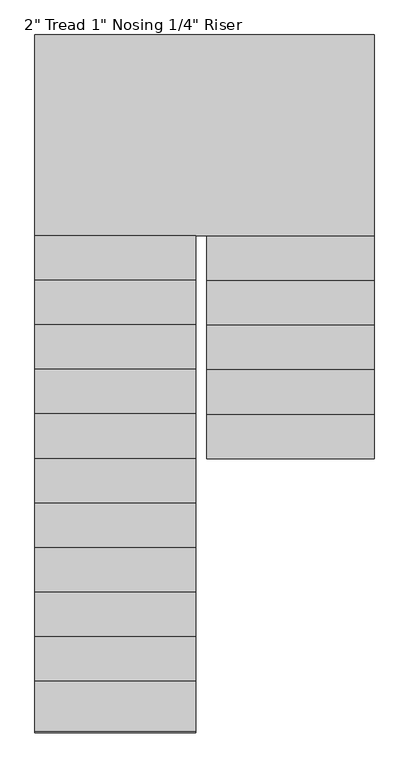
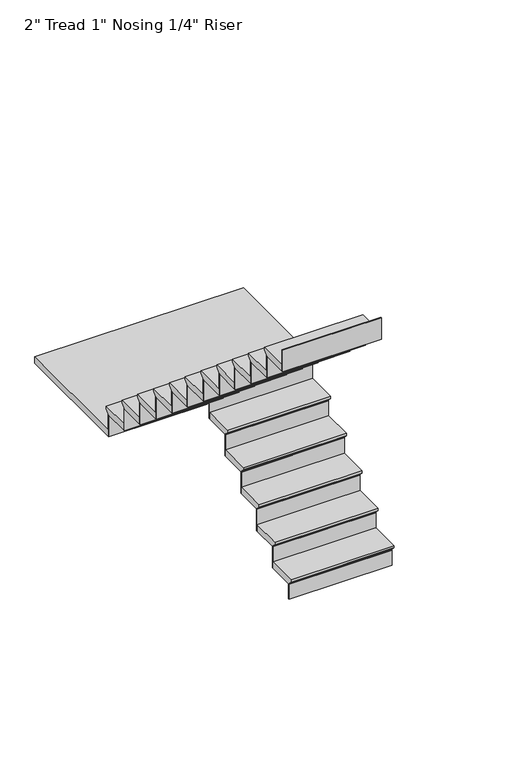
"""IFC4 building model written with IfcOpenShell, lengths in millimetres: stair flight geometry."""

from ifc_helpers import new_model, si_unit, origin, place, context, project, spatial, faceted_brep, source, transform, mapped, element, save


def stair_flight_e13e2030(model_context):
    return source(origin(), model_context, "Body", "Brep", [
        faceted_brep([(-3749.597125, 2714.6319226, 9141.8833333), (-3749.597125, 2714.6319226, 9160.9333333), (-4512.2136682, 2714.6319226, 9160.9333333), (-4512.2136682, 2714.6319226, 9141.8833333), (-3749.597125, 2740.0319226, 9116.4833333), (-4512.2136682, 2740.0319226, 9116.4833333), (-3749.597125, 2943.2319226, 9160.9333333), (-4512.2136682, 2943.2319226, 9160.9333333), (-4512.2136682, 2740.0319226, 9110.1333333), (-4512.2136682, 2943.2319226, 9110.1333333), (-3749.597125, 2943.2319226, 9110.1333333), (-3749.597125, 2740.0319226, 9110.1333333)], [[[0, 1, 2, 3]], [[4, 0, 3, 5]], [[2, 1, 6, 7]], [[8, 9, 10, 11]], [[2, 7, 9, 8, 5, 3]], [[8, 11, 4, 5]], [[6, 1, 0, 4, 11, 10]], [[7, 6, 10, 9]]]),
        faceted_brep([(-3749.597125, 2740.0319226, 9110.1333333), (-3749.597125, 2740.0319226, 8991.6), (-3749.597125, 2746.3819226, 8991.6), (-3749.597125, 2746.3819226, 9110.1333333), (-4512.2136682, 2740.0319226, 9110.1333333), (-4512.2136682, 2746.3819226, 9110.1333333), (-4512.2136682, 2746.3819226, 8991.6), (-4512.2136682, 2740.0319226, 8991.6)], [[[0, 1, 2, 3]], [[4, 5, 6, 7]], [[1, 0, 4, 7]], [[2, 1, 7, 6]], [[3, 2, 6, 5]], [[0, 3, 5, 4]]]),
        faceted_brep([(-3749.597125, 2943.2319226, 9279.4666667), (-3749.597125, 2943.2319226, 9110.1333333), (-3749.597125, 2949.5819226, 9110.1333333), (-3749.597125, 2949.5819226, 9279.4666667), (-4512.2136682, 2943.2319226, 9279.4666667), (-4512.2136682, 2949.5819226, 9279.4666667), (-4512.2136682, 2949.5819226, 9110.1333333), (-4512.2136682, 2943.2319226, 9110.1333333)], [[[0, 1, 2, 3]], [[4, 5, 6, 7]], [[1, 0, 4, 7]], [[2, 1, 7, 6]], [[3, 2, 6, 5]], [[0, 3, 5, 4]]]),
        faceted_brep([(-4512.2136682, 2917.8319226, 9330.2666667), (-3749.597125, 2917.8319226, 9330.2666667), (-3749.597125, 3146.4319226, 9330.2666667), (-4512.2136682, 3146.4319226, 9330.2666667), (-4512.2136682, 2943.2319226, 9279.4666667), (-4512.2136682, 3146.4319226, 9279.4666667), (-3749.597125, 3146.4319226, 9279.4666667), (-3749.597125, 2943.2319226, 9279.4666667), (-4512.2136682, 2943.2319226, 9285.8166667), (-4512.2136682, 2917.8319226, 9311.2166667), (-3749.597125, 2943.2319226, 9285.8166667), (-3749.597125, 2917.8319226, 9311.2166667)], [[[0, 1, 2, 3]], [[4, 5, 6, 7]], [[0, 3, 5, 4, 8, 9]], [[4, 7, 10, 8]], [[2, 1, 11, 10, 7, 6]], [[3, 2, 6, 5]], [[11, 1, 0, 9]], [[10, 11, 9, 8]]]),
        faceted_brep([(-3749.597125, 3146.4319226, 9448.8), (-3749.597125, 3146.4319226, 9279.4666667), (-3749.597125, 3152.7819226, 9279.4666667), (-3749.597125, 3152.7819226, 9448.8), (-4512.2136682, 3146.4319226, 9448.8), (-4512.2136682, 3152.7819226, 9448.8), (-4512.2136682, 3152.7819226, 9279.4666667), (-4512.2136682, 3146.4319226, 9279.4666667)], [[[0, 1, 2, 3]], [[4, 5, 6, 7]], [[1, 0, 4, 7]], [[2, 1, 7, 6]], [[3, 2, 6, 5]], [[0, 3, 5, 4]]]),
        faceted_brep([(-4512.2136682, 3121.0319226, 9499.6), (-3749.597125, 3121.0319226, 9499.6), (-3749.597125, 3349.6319226, 9499.6), (-4512.2136682, 3349.6319226, 9499.6), (-4512.2136682, 3146.4319226, 9448.8), (-4512.2136682, 3349.6319226, 9448.8), (-3749.597125, 3349.6319226, 9448.8), (-3749.597125, 3146.4319226, 9448.8), (-4512.2136682, 3146.4319226, 9455.15), (-4512.2136682, 3121.0319226, 9480.55), (-3749.597125, 3146.4319226, 9455.15), (-3749.597125, 3121.0319226, 9480.55)], [[[0, 1, 2, 3]], [[4, 5, 6, 7]], [[0, 3, 5, 4, 8, 9]], [[4, 7, 10, 8]], [[2, 1, 11, 10, 7, 6]], [[3, 2, 6, 5]], [[11, 1, 0, 9]], [[10, 11, 9, 8]]]),
        faceted_brep([(-3749.597125, 3349.6319226, 9618.1333333), (-3749.597125, 3349.6319226, 9448.8), (-3749.597125, 3355.9819226, 9448.8), (-3749.597125, 3355.9819226, 9618.1333333), (-4512.2136682, 3349.6319226, 9618.1333333), (-4512.2136682, 3355.9819226, 9618.1333333), (-4512.2136682, 3355.9819226, 9448.8), (-4512.2136682, 3349.6319226, 9448.8)], [[[0, 1, 2, 3]], [[4, 5, 6, 7]], [[1, 0, 4, 7]], [[2, 1, 7, 6]], [[3, 2, 6, 5]], [[0, 3, 5, 4]]]),
        faceted_brep([(-4512.2136682, 3324.2319226, 9668.9333333), (-3749.597125, 3324.2319226, 9668.9333333), (-3749.597125, 3552.8319226, 9668.9333333), (-4512.2136682, 3552.8319226, 9668.9333333), (-4512.2136682, 3349.6319226, 9618.1333333), (-4512.2136682, 3552.8319226, 9618.1333333), (-3749.597125, 3552.8319226, 9618.1333333), (-3749.597125, 3349.6319226, 9618.1333333), (-4512.2136682, 3349.6319226, 9624.4833333), (-4512.2136682, 3324.2319226, 9649.8833333), (-3749.597125, 3349.6319226, 9624.4833333), (-3749.597125, 3324.2319226, 9649.8833333)], [[[0, 1, 2, 3]], [[4, 5, 6, 7]], [[0, 3, 5, 4, 8, 9]], [[4, 7, 10, 8]], [[2, 1, 11, 10, 7, 6]], [[3, 2, 6, 5]], [[11, 1, 0, 9]], [[10, 11, 9, 8]]]),
        faceted_brep([(-3749.597125, 3552.8319226, 9787.4666667), (-3749.597125, 3552.8319226, 9618.1333333), (-3749.597125, 3559.1819226, 9618.1333333), (-3749.597125, 3559.1819226, 9787.4666667), (-4512.2136682, 3552.8319226, 9787.4666667), (-4512.2136682, 3559.1819226, 9787.4666667), (-4512.2136682, 3559.1819226, 9618.1333333), (-4512.2136682, 3552.8319226, 9618.1333333)], [[[0, 1, 2, 3]], [[4, 5, 6, 7]], [[1, 0, 4, 7]], [[2, 1, 7, 6]], [[3, 2, 6, 5]], [[0, 3, 5, 4]]]),
        faceted_brep([(-4512.2136682, 3527.4319226, 9838.2666667), (-3749.597125, 3527.4319226, 9838.2666667), (-3749.597125, 3756.0319226, 9838.2666667), (-4512.2136682, 3756.0319226, 9838.2666667), (-4512.2136682, 3552.8319226, 9787.4666667), (-4512.2136682, 3756.0319226, 9787.4666667), (-3749.597125, 3756.0319226, 9787.4666667), (-3749.597125, 3552.8319226, 9787.4666667), (-4512.2136682, 3552.8319226, 9793.8166667), (-4512.2136682, 3527.4319226, 9819.2166667), (-3749.597125, 3552.8319226, 9793.8166667), (-3749.597125, 3527.4319226, 9819.2166667)], [[[0, 1, 2, 3]], [[4, 5, 6, 7]], [[0, 3, 5, 4, 8, 9]], [[4, 7, 10, 8]], [[2, 1, 11, 10, 7, 6]], [[3, 2, 6, 5]], [[11, 1, 0, 9]], [[10, 11, 9, 8]]]),
        faceted_brep([(-3749.597125, 3756.0319226, 9956.8), (-3749.597125, 3756.0319226, 9787.4666667), (-3749.597125, 3762.3819226, 9787.4666667), (-3749.597125, 3762.3819226, 9956.8), (-4512.2136682, 3756.0319226, 9956.8), (-4512.2136682, 3762.3819226, 9956.8), (-4512.2136682, 3762.3819226, 9787.4666667), (-4512.2136682, 3756.0319226, 9787.4666667)], [[[0, 1, 2, 3]], [[4, 5, 6, 7]], [[1, 0, 4, 7]], [[2, 1, 7, 6]], [[3, 2, 6, 5]], [[0, 3, 5, 4]]]),
        faceted_brep([(-4563.0136682, 3705.2319226, 10007.6), (-4563.0136682, 3730.6319226, 10007.6), (-3749.597125, 3730.6319226, 10007.6), (-3749.597125, 4645.0319226, 10007.6), (-5295.0246464, 4645.0319226, 10007.6), (-5295.0246464, 3705.2319226, 10007.6), (-4563.0136682, 3730.6319226, 9956.8), (-4563.0136682, 3705.2319226, 9956.8), (-5295.0246464, 3705.2319226, 9956.8), (-5295.0246464, 4645.0319226, 9956.8), (-3749.597125, 4645.0319226, 9956.8), (-3749.597125, 3756.0319226, 9956.8), (-4512.2136682, 3756.0319226, 9956.8), (-4512.2136682, 3730.6319226, 9956.8), (-4512.2136682, 3730.6319226, 9988.55), (-3749.597125, 3730.6319226, 9988.55), (-4512.2136682, 3756.0319226, 9963.15), (-3749.597125, 3756.0319226, 9963.15)], [[[0, 1, 2, 3, 4, 5]], [[6, 7, 8, 9, 10, 11, 12, 13]], [[1, 0, 7, 6]], [[2, 1, 6, 13, 14, 15]], [[13, 12, 16, 14]], [[12, 11, 17, 16]], [[3, 2, 15, 17, 11, 10]], [[4, 3, 10, 9]], [[5, 4, 9, 8]], [[0, 5, 8, 7]], [[17, 15, 14, 16]]]),
        faceted_brep([(-5295.0246464, 3705.2319226, 10126.1333333), (-5295.0246464, 3705.2319226, 9956.8), (-5295.0246464, 3698.8819226, 9956.8), (-5295.0246464, 3698.8819226, 10126.1333333), (-4563.0136682, 3705.2319226, 10126.1333333), (-4563.0136682, 3698.8819226, 10126.1333333), (-4563.0136682, 3698.8819226, 9956.8), (-4563.0136682, 3705.2319226, 9956.8)], [[[0, 1, 2, 3]], [[4, 5, 6, 7]], [[1, 0, 4, 7]], [[2, 1, 7, 6]], [[3, 2, 6, 5]], [[0, 3, 5, 4]]]),
        faceted_brep([(-4563.0136682, 3730.6319226, 10176.9333333), (-5295.0246464, 3730.6319226, 10176.9333333), (-5295.0246464, 3502.0319226, 10176.9333333), (-4563.0136682, 3502.0319226, 10176.9333333), (-4563.0136682, 3705.2319226, 10126.1333333), (-4563.0136682, 3502.0319226, 10126.1333333), (-5295.0246464, 3502.0319226, 10126.1333333), (-5295.0246464, 3705.2319226, 10126.1333333), (-4563.0136682, 3705.2319226, 10132.4833333), (-4563.0136682, 3730.6319226, 10157.8833333), (-5295.0246464, 3705.2319226, 10132.4833333), (-5295.0246464, 3730.6319226, 10157.8833333)], [[[0, 1, 2, 3]], [[4, 5, 6, 7]], [[0, 3, 5, 4, 8, 9]], [[4, 7, 10, 8]], [[2, 1, 11, 10, 7, 6]], [[3, 2, 6, 5]], [[11, 1, 0, 9]], [[10, 11, 9, 8]]]),
        faceted_brep([(-5295.0246464, 3502.0319226, 10295.4666667), (-5295.0246464, 3502.0319226, 10126.1333333), (-5295.0246464, 3495.6819226, 10126.1333333), (-5295.0246464, 3495.6819226, 10295.4666667), (-4563.0136682, 3502.0319226, 10295.4666667), (-4563.0136682, 3495.6819226, 10295.4666667), (-4563.0136682, 3495.6819226, 10126.1333333), (-4563.0136682, 3502.0319226, 10126.1333333)], [[[0, 1, 2, 3]], [[4, 5, 6, 7]], [[1, 0, 4, 7]], [[2, 1, 7, 6]], [[3, 2, 6, 5]], [[0, 3, 5, 4]]]),
        faceted_brep([(-4563.0136682, 3527.4319226, 10346.2666667), (-5295.0246464, 3527.4319226, 10346.2666667), (-5295.0246464, 3298.8319226, 10346.2666667), (-4563.0136682, 3298.8319226, 10346.2666667), (-4563.0136682, 3502.0319226, 10295.4666667), (-4563.0136682, 3298.8319226, 10295.4666667), (-5295.0246464, 3298.8319226, 10295.4666667), (-5295.0246464, 3502.0319226, 10295.4666667), (-4563.0136682, 3502.0319226, 10301.8166667), (-4563.0136682, 3527.4319226, 10327.2166667), (-5295.0246464, 3502.0319226, 10301.8166667), (-5295.0246464, 3527.4319226, 10327.2166667)], [[[0, 1, 2, 3]], [[4, 5, 6, 7]], [[0, 3, 5, 4, 8, 9]], [[4, 7, 10, 8]], [[2, 1, 11, 10, 7, 6]], [[3, 2, 6, 5]], [[11, 1, 0, 9]], [[10, 11, 9, 8]]]),
        faceted_brep([(-5295.0246464, 3298.8319226, 10464.8), (-5295.0246464, 3298.8319226, 10295.4666667), (-5295.0246464, 3292.4819226, 10295.4666667), (-5295.0246464, 3292.4819226, 10464.8), (-4563.0136682, 3298.8319226, 10464.8), (-4563.0136682, 3292.4819226, 10464.8), (-4563.0136682, 3292.4819226, 10295.4666667), (-4563.0136682, 3298.8319226, 10295.4666667)], [[[0, 1, 2, 3]], [[4, 5, 6, 7]], [[1, 0, 4, 7]], [[2, 1, 7, 6]], [[3, 2, 6, 5]], [[0, 3, 5, 4]]]),
        faceted_brep([(-4563.0136682, 3324.2319226, 10515.6), (-5295.0246464, 3324.2319226, 10515.6), (-5295.0246464, 3095.6319226, 10515.6), (-4563.0136682, 3095.6319226, 10515.6), (-4563.0136682, 3298.8319226, 10464.8), (-4563.0136682, 3095.6319226, 10464.8), (-5295.0246464, 3095.6319226, 10464.8), (-5295.0246464, 3298.8319226, 10464.8), (-4563.0136682, 3298.8319226, 10471.15), (-4563.0136682, 3324.2319226, 10496.55), (-5295.0246464, 3298.8319226, 10471.15), (-5295.0246464, 3324.2319226, 10496.55)], [[[0, 1, 2, 3]], [[4, 5, 6, 7]], [[0, 3, 5, 4, 8, 9]], [[4, 7, 10, 8]], [[2, 1, 11, 10, 7, 6]], [[3, 2, 6, 5]], [[11, 1, 0, 9]], [[10, 11, 9, 8]]]),
        faceted_brep([(-5295.0246464, 3095.6319226, 10634.1333333), (-5295.0246464, 3095.6319226, 10464.8), (-5295.0246464, 3089.2819226, 10464.8), (-5295.0246464, 3089.2819226, 10634.1333333), (-4563.0136682, 3095.6319226, 10634.1333333), (-4563.0136682, 3089.2819226, 10634.1333333), (-4563.0136682, 3089.2819226, 10464.8), (-4563.0136682, 3095.6319226, 10464.8)], [[[0, 1, 2, 3]], [[4, 5, 6, 7]], [[1, 0, 4, 7]], [[2, 1, 7, 6]], [[3, 2, 6, 5]], [[0, 3, 5, 4]]]),
        faceted_brep([(-4563.0136682, 3121.0319226, 10684.9333333), (-5295.0246464, 3121.0319226, 10684.9333333), (-5295.0246464, 2892.4319226, 10684.9333333), (-4563.0136682, 2892.4319226, 10684.9333333), (-4563.0136682, 3095.6319226, 10634.1333333), (-4563.0136682, 2892.4319226, 10634.1333333), (-5295.0246464, 2892.4319226, 10634.1333333), (-5295.0246464, 3095.6319226, 10634.1333333), (-4563.0136682, 3095.6319226, 10640.4833333), (-4563.0136682, 3121.0319226, 10665.8833333), (-5295.0246464, 3095.6319226, 10640.4833333), (-5295.0246464, 3121.0319226, 10665.8833333)], [[[0, 1, 2, 3]], [[4, 5, 6, 7]], [[0, 3, 5, 4, 8, 9]], [[4, 7, 10, 8]], [[2, 1, 11, 10, 7, 6]], [[3, 2, 6, 5]], [[11, 1, 0, 9]], [[10, 11, 9, 8]]]),
        faceted_brep([(-5295.0246464, 2892.4319226, 10803.4666667), (-5295.0246464, 2892.4319226, 10634.1333333), (-5295.0246464, 2886.0819226, 10634.1333333), (-5295.0246464, 2886.0819226, 10803.4666667), (-4563.0136682, 2892.4319226, 10803.4666667), (-4563.0136682, 2886.0819226, 10803.4666667), (-4563.0136682, 2886.0819226, 10634.1333333), (-4563.0136682, 2892.4319226, 10634.1333333)], [[[0, 1, 2, 3]], [[4, 5, 6, 7]], [[1, 0, 4, 7]], [[2, 1, 7, 6]], [[3, 2, 6, 5]], [[0, 3, 5, 4]]]),
        faceted_brep([(-4563.0136682, 2917.8319226, 10854.2666667), (-5295.0246464, 2917.8319226, 10854.2666667), (-5295.0246464, 2689.2319226, 10854.2666667), (-4563.0136682, 2689.2319226, 10854.2666667), (-4563.0136682, 2892.4319226, 10803.4666667), (-4563.0136682, 2689.2319226, 10803.4666667), (-5295.0246464, 2689.2319226, 10803.4666667), (-5295.0246464, 2892.4319226, 10803.4666667), (-4563.0136682, 2892.4319226, 10809.8166667), (-4563.0136682, 2917.8319226, 10835.2166667), (-5295.0246464, 2892.4319226, 10809.8166667), (-5295.0246464, 2917.8319226, 10835.2166667)], [[[0, 1, 2, 3]], [[4, 5, 6, 7]], [[0, 3, 5, 4, 8, 9]], [[4, 7, 10, 8]], [[2, 1, 11, 10, 7, 6]], [[3, 2, 6, 5]], [[11, 1, 0, 9]], [[10, 11, 9, 8]]]),
        faceted_brep([(-5295.0246464, 2689.2319226, 10972.8), (-5295.0246464, 2689.2319226, 10803.4666667), (-5295.0246464, 2682.8819226, 10803.4666667), (-5295.0246464, 2682.8819226, 10972.8), (-4563.0136682, 2689.2319226, 10972.8), (-4563.0136682, 2682.8819226, 10972.8), (-4563.0136682, 2682.8819226, 10803.4666667), (-4563.0136682, 2689.2319226, 10803.4666667)], [[[0, 1, 2, 3]], [[4, 5, 6, 7]], [[1, 0, 4, 7]], [[2, 1, 7, 6]], [[3, 2, 6, 5]], [[0, 3, 5, 4]]]),
        faceted_brep([(-4563.0136682, 2714.6319226, 11023.6), (-5295.0246464, 2714.6319226, 11023.6), (-5295.0246464, 2486.0319226, 11023.6), (-4563.0136682, 2486.0319226, 11023.6), (-4563.0136682, 2689.2319226, 10972.8), (-4563.0136682, 2486.0319226, 10972.8), (-5295.0246464, 2486.0319226, 10972.8), (-5295.0246464, 2689.2319226, 10972.8), (-4563.0136682, 2689.2319226, 10979.15), (-4563.0136682, 2714.6319226, 11004.55), (-5295.0246464, 2689.2319226, 10979.15), (-5295.0246464, 2714.6319226, 11004.55)], [[[0, 1, 2, 3]], [[4, 5, 6, 7]], [[0, 3, 5, 4, 8, 9]], [[4, 7, 10, 8]], [[2, 1, 11, 10, 7, 6]], [[3, 2, 6, 5]], [[11, 1, 0, 9]], [[10, 11, 9, 8]]]),
        faceted_brep([(-5295.0246464, 2486.0319226, 11142.1333333), (-5295.0246464, 2486.0319226, 10972.8), (-5295.0246464, 2479.6819226, 10972.8), (-5295.0246464, 2479.6819226, 11142.1333333), (-4563.0136682, 2486.0319226, 11142.1333333), (-4563.0136682, 2479.6819226, 11142.1333333), (-4563.0136682, 2479.6819226, 10972.8), (-4563.0136682, 2486.0319226, 10972.8)], [[[0, 1, 2, 3]], [[4, 5, 6, 7]], [[1, 0, 4, 7]], [[2, 1, 7, 6]], [[3, 2, 6, 5]], [[0, 3, 5, 4]]]),
        faceted_brep([(-4563.0136682, 2511.4319226, 11192.9333333), (-5295.0246464, 2511.4319226, 11192.9333333), (-5295.0246464, 2282.8319226, 11192.9333333), (-4563.0136682, 2282.8319226, 11192.9333333), (-4563.0136682, 2486.0319226, 11142.1333333), (-4563.0136682, 2282.8319226, 11142.1333333), (-5295.0246464, 2282.8319226, 11142.1333333), (-5295.0246464, 2486.0319226, 11142.1333333), (-4563.0136682, 2486.0319226, 11148.4833333), (-4563.0136682, 2511.4319226, 11173.8833333), (-5295.0246464, 2486.0319226, 11148.4833333), (-5295.0246464, 2511.4319226, 11173.8833333)], [[[0, 1, 2, 3]], [[4, 5, 6, 7]], [[0, 3, 5, 4, 8, 9]], [[4, 7, 10, 8]], [[2, 1, 11, 10, 7, 6]], [[3, 2, 6, 5]], [[11, 1, 0, 9]], [[10, 11, 9, 8]]]),
        faceted_brep([(-5295.0246464, 2282.8319226, 11311.4666667), (-5295.0246464, 2282.8319226, 11142.1333333), (-5295.0246464, 2276.4819226, 11142.1333333), (-5295.0246464, 2276.4819226, 11311.4666667), (-4563.0136682, 2282.8319226, 11311.4666667), (-4563.0136682, 2276.4819226, 11311.4666667), (-4563.0136682, 2276.4819226, 11142.1333333), (-4563.0136682, 2282.8319226, 11142.1333333)], [[[0, 1, 2, 3]], [[4, 5, 6, 7]], [[1, 0, 4, 7]], [[2, 1, 7, 6]], [[3, 2, 6, 5]], [[0, 3, 5, 4]]]),
        faceted_brep([(-4563.0136682, 2308.2319226, 11362.2666667), (-5295.0246464, 2308.2319226, 11362.2666667), (-5295.0246464, 2079.6319226, 11362.2666667), (-4563.0136682, 2079.6319226, 11362.2666667), (-4563.0136682, 2282.8319226, 11311.4666667), (-4563.0136682, 2079.6319226, 11311.4666667), (-5295.0246464, 2079.6319226, 11311.4666667), (-5295.0246464, 2282.8319226, 11311.4666667), (-4563.0136682, 2282.8319226, 11317.8166667), (-4563.0136682, 2308.2319226, 11343.2166667), (-5295.0246464, 2282.8319226, 11317.8166667), (-5295.0246464, 2308.2319226, 11343.2166667)], [[[0, 1, 2, 3]], [[4, 5, 6, 7]], [[0, 3, 5, 4, 8, 9]], [[4, 7, 10, 8]], [[2, 1, 11, 10, 7, 6]], [[3, 2, 6, 5]], [[11, 1, 0, 9]], [[10, 11, 9, 8]]]),
        faceted_brep([(-5295.0246464, 2079.6319226, 11480.8), (-5295.0246464, 2079.6319226, 11311.4666667), (-5295.0246464, 2073.2819226, 11311.4666667), (-5295.0246464, 2073.2819226, 11480.8), (-4563.0136682, 2079.6319226, 11480.8), (-4563.0136682, 2073.2819226, 11480.8), (-4563.0136682, 2073.2819226, 11311.4666667), (-4563.0136682, 2079.6319226, 11311.4666667)], [[[0, 1, 2, 3]], [[4, 5, 6, 7]], [[1, 0, 4, 7]], [[2, 1, 7, 6]], [[3, 2, 6, 5]], [[0, 3, 5, 4]]]),
        faceted_brep([(-4563.0136682, 2105.0319226, 11531.6), (-5295.0246464, 2105.0319226, 11531.6), (-5295.0246464, 1876.4319226, 11531.6), (-4563.0136682, 1876.4319226, 11531.6), (-4563.0136682, 2079.6319226, 11480.8), (-4563.0136682, 1876.4319226, 11480.8), (-5295.0246464, 1876.4319226, 11480.8), (-5295.0246464, 2079.6319226, 11480.8), (-4563.0136682, 2079.6319226, 11487.15), (-4563.0136682, 2105.0319226, 11512.55), (-5295.0246464, 2079.6319226, 11487.15), (-5295.0246464, 2105.0319226, 11512.55)], [[[0, 1, 2, 3]], [[4, 5, 6, 7]], [[0, 3, 5, 4, 8, 9]], [[4, 7, 10, 8]], [[2, 1, 11, 10, 7, 6]], [[3, 2, 6, 5]], [[11, 1, 0, 9]], [[10, 11, 9, 8]]]),
        faceted_brep([(-5295.0246464, 1876.4319226, 11650.1333333), (-5295.0246464, 1876.4319226, 11480.8), (-5295.0246464, 1870.0819226, 11480.8), (-5295.0246464, 1870.0819226, 11650.1333333), (-4563.0136682, 1876.4319226, 11650.1333333), (-4563.0136682, 1870.0819226, 11650.1333333), (-4563.0136682, 1870.0819226, 11480.8), (-4563.0136682, 1876.4319226, 11480.8)], [[[0, 1, 2, 3]], [[4, 5, 6, 7]], [[1, 0, 4, 7]], [[2, 1, 7, 6]], [[3, 2, 6, 5]], [[0, 3, 5, 4]]]),
        faceted_brep([(-4563.0136682, 1901.8319226, 11700.9333333), (-5295.0246464, 1901.8319226, 11700.9333333), (-5295.0246464, 1673.2319226, 11700.9333333), (-4563.0136682, 1673.2319226, 11700.9333333), (-4563.0136682, 1876.4319226, 11650.1333333), (-4563.0136682, 1673.2319226, 11650.1333333), (-5295.0246464, 1673.2319226, 11650.1333333), (-5295.0246464, 1876.4319226, 11650.1333333), (-4563.0136682, 1876.4319226, 11656.4833333), (-4563.0136682, 1901.8319226, 11681.8833333), (-5295.0246464, 1876.4319226, 11656.4833333), (-5295.0246464, 1901.8319226, 11681.8833333)], [[[0, 1, 2, 3]], [[4, 5, 6, 7]], [[0, 3, 5, 4, 8, 9]], [[4, 7, 10, 8]], [[2, 1, 11, 10, 7, 6]], [[3, 2, 6, 5]], [[11, 1, 0, 9]], [[10, 11, 9, 8]]]),
        faceted_brep([(-5295.0246464, 1673.2319226, 11819.4666667), (-5295.0246464, 1673.2319226, 11650.1333333), (-5295.0246464, 1666.8819226, 11650.1333333), (-5295.0246464, 1666.8819226, 11819.4666667), (-4563.0136682, 1673.2319226, 11819.4666667), (-4563.0136682, 1666.8819226, 11819.4666667), (-4563.0136682, 1666.8819226, 11650.1333333), (-4563.0136682, 1673.2319226, 11650.1333333)], [[[0, 1, 2, 3]], [[4, 5, 6, 7]], [[1, 0, 4, 7]], [[2, 1, 7, 6]], [[3, 2, 6, 5]], [[0, 3, 5, 4]]]),
        faceted_brep([(-4563.0136682, 1698.6319226, 11870.2666667), (-5295.0246464, 1698.6319226, 11870.2666667), (-5295.0246464, 1470.0319226, 11870.2666667), (-4563.0136682, 1470.0319226, 11870.2666667), (-4563.0136682, 1673.2319226, 11819.4666667), (-4563.0136682, 1470.0319226, 11819.4666667), (-5295.0246464, 1470.0319226, 11819.4666667), (-5295.0246464, 1673.2319226, 11819.4666667), (-4563.0136682, 1673.2319226, 11825.8166667), (-4563.0136682, 1698.6319226, 11851.2166667), (-5295.0246464, 1673.2319226, 11825.8166667), (-5295.0246464, 1698.6319226, 11851.2166667)], [[[0, 1, 2, 3]], [[4, 5, 6, 7]], [[0, 3, 5, 4, 8, 9]], [[4, 7, 10, 8]], [[2, 1, 11, 10, 7, 6]], [[3, 2, 6, 5]], [[11, 1, 0, 9]], [[10, 11, 9, 8]]]),
        faceted_brep([(-5295.0246464, 1470.0319226, 11988.8), (-5295.0246464, 1470.0319226, 11819.4666667), (-5295.0246464, 1463.6819226, 11819.4666667), (-5295.0246464, 1463.6819226, 11988.8), (-4563.0136682, 1470.0319226, 11988.8), (-4563.0136682, 1463.6819226, 11988.8), (-4563.0136682, 1463.6819226, 11819.4666667), (-4563.0136682, 1470.0319226, 11819.4666667)], [[[0, 1, 2, 3]], [[4, 5, 6, 7]], [[1, 0, 4, 7]], [[2, 1, 7, 6]], [[3, 2, 6, 5]], [[0, 3, 5, 4]]]),
    ])


if __name__ == "__main__":
    model = new_model("IFC4")
    model_context = context("Model", 3, world=origin())
    ifc_project = project(units=[si_unit("LENGTHUNIT", "METRE", prefix="MILLI")], contexts=[model_context])
    site = spatial("IfcSite", under=ifc_project)
    building = spatial("IfcBuilding", under=site)
    placement = place(None, origin())
    stair_flight_shape = stair_flight_e13e2030(model_context)
    element("IfcStairFlight", 1, ObjectType="2\" Tread 1\" Nosing 1/4\" Riser", at=placement, inside=building, context=model_context, shape_type="MappedRepresentation", body=[
        mapped(stair_flight_shape, transform((0.0, 0.0, 0.0), x_axis=(1.0, 0.0, 0.0), y_axis=(0.0, 1.0, 0.0), z_axis=(0.0, 0.0, 1.0))),
    ])
    save(model, "model.ifc")
